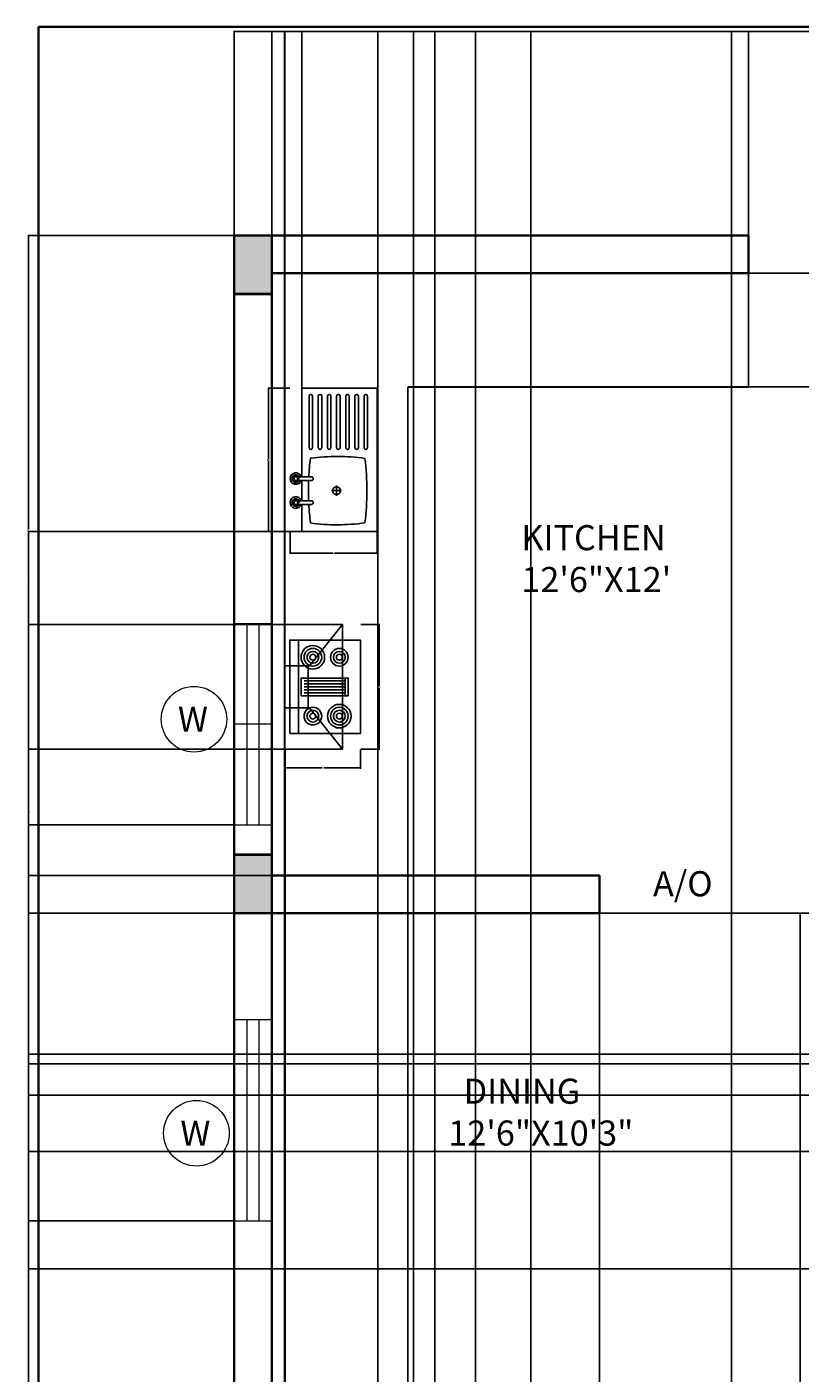
# Model space of a CAD drawing. Units: inches. Extents: x 2243 to 2668, y 14541 to 15226.
# Tile 3 of 5: x 2243 to 2428, y 14904 to 15226. Entities that reach past the tile are written whole.
import ezdxf

# ---------------------------------------------------------------- set-up
doc = ezdxf.new("R2010")
doc.units = ezdxf.units.IN
doc.header["$MEASUREMENT"] = 0
for name, color, linetype, lineweight in [('A-ANNO-DIMS', 2, 'Continuous', 18), ('A-ANNO-SYMB', 3, 'Continuous', 18), ('A-ANNO-TTLB', 7, 'Continuous', 35), ('A-AREA-IDEN', 7, 'Continuous', 18), ('A-COLS', 7, 'Continuous', 40), ('A-COLS-PATT', 7, 'Continuous', 13), ('A-EQPM', 8, 'Continuous', 25), ('A-FLOR-CASE', 9, 'Continuous', 25), ('A-FLOR-FIXT', 8, 'Continuous', 25), ('A-GLAZ', 4, 'Continuous', 18), ('A-WALL', 7, 'Continuous', 35)]:
    doc.layers.add(name, color=color, linetype=linetype, lineweight=lineweight)
doc.styles.get("Standard").update_dxf_attribs({"font": 'arial.ttf'})
doc.dimstyles.get("Standard").update_dxf_attribs({"dimtxt": 0.18, "dimasz": 0.18, "dimexe": 0.18, "dimexo": 0.0625, "dimgap": 0.09, "dimtad": 0, "dimtih": 1, "dimtoh": 1, "dimdec": 4, "dimzin": 0, "dimdsep": 46, "dimtxsty": 'Standard', "dimcen": 0.09, "dimadec": 0, "dimazin": 0, "dimtfac": 1, "dimtdec": 4, "dimtofl": 0, "dimtmove": 0, "dimatfit": 3, "dimfxl": 1, "dimtolj": 1, "dimtzin": 0, "dimarcsym": 0})

# ---------------------------------------------------------------- blocks, each defined once
blk = doc.blocks.new('chimmne')
for p, q in [((17.89, 6.07), (-18.11, 6.07)), ((-18.11, 6.07), (-18.11, -10.43)), ((-6.16, -3.43), (-18.11, 6.07)), ((5.94, -3.43), (17.89, 6.07)), ((17.89, 6.07), (17.89, -10.43)), ((-6.16, -3.43), (-6.16, -10.43)), ((5.94, -3.82), (-6.16, -3.82)), ((5.94, -3.43), (5.94, -10.43))]:
    blk.add_line(p, q)
for points in [[(-13.61, -9.12), (-13.61, 11.28), (13.39, 11.28), (13.39, -9.12)], [(-2.66, -5.87), (-2.66, 7.73), (2.44, 7.73), (2.44, -5.87)]]:
    blk.add_lwpolyline(points, close=True)
for points in [[(-2.66, 6.88), (2.44, 6.88)], [(-1.81, 6.88), (-1.81, -5.02)], [(-0.96, -5.02), (-0.96, 6.88)], [(-0.11, 6.88), (-0.11, -5.02)], [(0.74, -5.02), (0.74, 6.88)], [(1.59, 6.88), (1.59, -5.02)], [(13.39, -6.57), (-13.61, -6.57)]]:
    blk.add_lwpolyline(points)
for centre, radius in [((-8.55, 5.18), 3.4), ((-8.55, 5.18), 2.55), ((-8.55, 5.18), 1.7), ((-8.55, 5.18), 0.85), ((8.44, 5.18), 2.55), ((8.44, 5.18), 1.7), ((8.44, 5.18), 0.85), ((-8.55, -2.47), 2.55), ((8.44, -2.47), 3.4), ((8.44, -2.47), 2.55), ((-8.55, -2.47), 1.7), ((-8.55, -2.47), 0.85), ((8.44, -2.47), 1.7), ((8.44, -2.47), 0.85)]:
    blk.add_circle(centre, radius)
blk = doc.blocks.new('A$C799204C7')
for p, q in [((0, 34.2), (17.99, 34.2)), ((0, 0), (0, 34.2)), ((2.32, 20.01), (2.32, 32.27)), ((3.13, 20.01), (3.13, 32.27)), ((4.48, 20.01), (4.48, 32.27)), ((5.29, 20.01), (5.29, 32.27)), ((6.64, 20.01), (6.64, 32.27)), ((7.45, 20.01), (7.45, 32.27)), ((8.85, 20.01), (8.85, 32.27)), ((9.66, 20.01), (9.66, 32.27)), ((11.01, 20.01), (11.01, 32.27)), ((11.82, 20.01), (11.82, 32.27)), ((13.22, 20.01), (13.22, 32.27)), ((14.03, 20.01), (14.03, 32.27)), ((15.42, 20.01), (15.42, 32.27)), ((16.24, 20.01), (16.24, 32.27)), ((17.99, 13.08), (17.99, 34.2)), ((18.59, 13.08), (15.71, 13.08)), ((8.52, 9.77), (10.9, 9.77)), ((9.73, 11), (9.73, 8.54)), ((15.71, 12.17), (18.59, 12.17)), ((17.99, 7.36), (17.99, 12.17)), ((18.59, 7.36), (15.71, 7.36)), ((15.71, 6.45), (18.59, 6.45)), ((17.99, 0), (17.99, 6.45)), ((0, 0), (17.99, 0))]:
    blk.add_line(p, q)
for centre, radius in [((19.38, 12.62), 0.684), ((19.38, 12.62), 0.456), ((9.7, 9.77), 0.916), ((19.38, 6.91), 0.684), ((19.38, 6.91), 0.456)]:
    blk.add_circle(centre, radius)
for centre, radius, start, end in [((2.72, 32.27), 0.407, 0, 180), ((4.88, 32.27), 0.407, 0, 180), ((7.05, 32.27), 0.407, 0, 180), ((9.25, 32.27), 0.407, 0, 180), ((11.42, 32.27), 0.407, 0, 180), ((13.62, 32.27), 0.407, 0, 180), ((15.83, 32.27), 0.407, 0, 180), ((2.72, 20.01), 0.407, 180, 0), ((4.88, 20.01), 0.407, 180, 0), ((7.05, 20.01), 0.407, 180, 0), ((9.25, 20.01), 0.407, 180, 0), ((11.42, 20.01), 0.407, 180, 0), ((13.62, 20.01), 0.407, 180, 0), ((15.83, 20.01), 0.407, 180, 0), ((67.33, 9.77), 64.88, 173.1952, 186.8048), ((9.53, -30.19), 48.1, 82.3437, 97.8966), ((-48.51, 9.77), 64.88, 2.9208, 6.8048), ((15.71, 12.62), 0.456, 90, 270), ((19.38, 12.62), 1.37, 199.6514, 160.3603), ((19.38, 12.62), 0.911, 210.3431, 149.7554), ((-48.51, 9.77), 64.88, 357.8723, 2.115), ((15.71, 6.91), 0.456, 90, 270), ((-48.51, 9.77), 64.88, 353.1952, 357.0665), ((19.38, 6.91), 1.37, 199.6514, 160.3603), ((19.38, 6.91), 0.911, 210.3431, 149.7554), ((9.53, 49.73), 48.1, 262.1034, 277.6563)]:
    blk.add_arc(centre, radius, start, end)
blk = doc.blocks.new('WIN-48IN')
for p, q in [((0, 9), (0, 0)), ((48, 9), (0, 9)), ((48, 0), (48, 9)), ((48, 6), (0, 6)), ((0, 3), (48, 3)), ((0, 0), (48, 0))]:
    blk.add_line(p, q)
blk = doc.blocks.new('TAG-WINDOW-W')
blk.add_circle((7.84, 7.84), 7.84)
at = {"insert": (3.99, 10.84), "char_height": 6, "attachment_point": 1}
blk.add_mtext_dynamic_manual_height_columns('W', width=14.3449, gutter_width=30, heights=[0], dxfattribs=at)
blk = doc.blocks.new('*D13')
at = {"layer": 'A-ANNO-DIMS', "color": 0, "lineweight": -2, "transparency": 16777216}
for p, q in [((2323.21, 15083.13), (2327.79, 15083.13)), ((2327.61, 15082.95), (2327.61, 15068.41)), ((2327.61, 15053.5), (2327.61, 15068.04)), ((2323.21, 15053.32), (2327.79, 15053.32))]:
    blk.add_line(p, q, dxfattribs=at)
at = {"layer": 'A-ANNO-DIMS', "color": 0, "transparency": 16777216}
for points in [[(2327.58, 15082.95), (2327.64, 15082.95), (2327.61, 15083.13)], [(2327.58, 15053.5), (2327.64, 15053.5), (2327.61, 15053.32)]]:
    blk.add_solid(points, dxfattribs=at)
at = {"layer": 'Defpoints', "color": 0, "transparency": 16777216}
for p in [(2323.14, 15083.13), (2327.61, 15083.13), (2323.14, 15053.32)]:
    blk.add_point(p, dxfattribs=at)
at = {"layer": 'A-ANNO-DIMS', "color": 0, "transparency": 16777216, "insert": (2327.61, 15068.23), "char_height": 0.18, "attachment_point": 5}
blk.add_mtext('\\A1;HOB 30', dxfattribs=at)
blk = doc.blocks.new('*D14')
at = {"layer": 'A-ANNO-DIMS', "color": 0, "lineweight": -2, "transparency": 16777216}
for p, q in [((2305.17, 15053.26), (2305.17, 15048.67)), ((2323.14, 15053.26), (2323.14, 15048.67)), ((2305.35, 15048.85), (2313.95, 15048.85)), ((2322.96, 15048.85), (2314.37, 15048.85))]:
    blk.add_line(p, q, dxfattribs=at)
at = {"layer": 'A-ANNO-DIMS', "color": 0, "transparency": 16777216}
for points in [[(2305.35, 15048.88), (2305.35, 15048.82), (2305.17, 15048.85)], [(2322.96, 15048.88), (2322.96, 15048.82), (2323.14, 15048.85)]]:
    blk.add_solid(points, dxfattribs=at)
at = {"layer": 'Defpoints', "color": 0, "transparency": 16777216}
for p in [(2305.17, 15053.32), (2323.14, 15053.32), (2323.14, 15048.85)]:
    blk.add_point(p, dxfattribs=at)
at = {"layer": 'A-ANNO-DIMS', "color": 0, "transparency": 16777216, "insert": (2314.16, 15048.85), "char_height": 0.18, "attachment_point": 5}
blk.add_mtext('\\A1;18', dxfattribs=at)
blk = doc.blocks.new('*D15')
at = {"layer": 'A-ANNO-DIMS', "color": 0, "lineweight": -2, "transparency": 16777216}
for p, q in [((2306.26, 15139.64), (2301, 15139.64)), ((2301.18, 15139.46), (2301.18, 15122.67)), ((2301.18, 15105.51), (2301.18, 15122.3)), ((2306.26, 15105.33), (2301, 15105.33))]:
    blk.add_line(p, q, dxfattribs=at)
at = {"layer": 'A-ANNO-DIMS', "color": 0, "transparency": 16777216}
for points in [[(2301.15, 15139.46), (2301.21, 15139.46), (2301.18, 15139.64)], [(2301.15, 15105.51), (2301.21, 15105.51), (2301.18, 15105.33)]]:
    blk.add_solid(points, dxfattribs=at)
at = {"layer": 'Defpoints', "color": 0, "transparency": 16777216}
for p in [(2301.18, 15139.64), (2306.32, 15139.64), (2306.32, 15105.33)]:
    blk.add_point(p, dxfattribs=at)
at = {"layer": 'A-ANNO-DIMS', "color": 0, "transparency": 16777216, "insert": (2301.18, 15122.49), "char_height": 0.18, "attachment_point": 5}
blk.add_mtext('\\A1;SINK 34', dxfattribs=at)
blk = doc.blocks.new('*D16')
at = {"layer": 'A-ANNO-DIMS', "color": 0, "lineweight": -2, "transparency": 16777216}
for p, q in [((2306.32, 15105.27), (2306.32, 15100.01)), ((2327.14, 15105.27), (2327.14, 15100.01)), ((2306.5, 15100.19), (2316.53, 15100.19)), ((2326.96, 15100.19), (2316.93, 15100.19))]:
    blk.add_line(p, q, dxfattribs=at)
at = {"layer": 'A-ANNO-DIMS', "color": 0, "transparency": 16777216}
for points in [[(2306.5, 15100.22), (2306.5, 15100.16), (2306.32, 15100.19)], [(2326.96, 15100.22), (2326.96, 15100.16), (2327.14, 15100.19)]]:
    blk.add_solid(points, dxfattribs=at)
at = {"layer": 'Defpoints', "color": 0, "transparency": 16777216}
for p in [(2306.32, 15105.33), (2327.14, 15105.33), (2306.32, 15100.19)]:
    blk.add_point(p, dxfattribs=at)
at = {"layer": 'A-ANNO-DIMS', "color": 0, "transparency": 16777216, "insert": (2316.73, 15100.19), "char_height": 0.18, "attachment_point": 5}
blk.add_mtext('\\A1;21', dxfattribs=at)
blk = doc.blocks.new('*D17')
at = {"layer": 'A-ANNO-DIMS', "color": 0, "lineweight": -2, "transparency": 16777216}
for p, q in [((2292.96, 15176.2), (2292.96, 15225.04)), ((2293.14, 15224.86), (2448.67, 15224.86)), ((2604.78, 15224.86), (2449.25, 15224.86)), ((2604.96, 15176.2), (2604.96, 15225.04))]:
    blk.add_line(p, q, dxfattribs=at)
at = {"layer": 'A-ANNO-DIMS', "color": 0, "transparency": 16777216}
for points in [[(2293.14, 15224.89), (2293.14, 15224.83), (2292.96, 15224.86)], [(2604.78, 15224.89), (2604.78, 15224.83), (2604.96, 15224.86)]]:
    blk.add_solid(points, dxfattribs=at)
at = {"layer": 'Defpoints', "color": 0, "transparency": 16777216}
for p in [(2604.96, 15224.86), (2292.96, 15176.14), (2604.96, 15176.14)]:
    blk.add_point(p, dxfattribs=at)
at = {"layer": 'A-ANNO-DIMS', "color": 0, "transparency": 16777216, "insert": (2448.96, 15224.86), "char_height": 0.18, "attachment_point": 5}
blk.add_mtext('\\A1;312', dxfattribs=at)
blk = doc.blocks.new('*D25')
at = {"layer": 'A-ANNO-DIMS', "color": 0, "lineweight": -2, "transparency": 16777216}
for p, q in [((2292.9, 14940.64), (2243.57, 14940.64)), ((2243.75, 14940.46), (2243.75, 14909.07)), ((2243.75, 14877.32), (2243.75, 14908.71)), ((2292.9, 14877.14), (2243.57, 14877.14))]:
    blk.add_line(p, q, dxfattribs=at)
at = {"layer": 'A-ANNO-DIMS', "color": 0, "transparency": 16777216}
for points in [[(2243.72, 14940.46), (2243.78, 14940.46), (2243.75, 14940.64)], [(2243.72, 14877.32), (2243.78, 14877.32), (2243.75, 14877.14)]]:
    blk.add_solid(points, dxfattribs=at)
at = {"layer": 'Defpoints', "color": 0, "transparency": 16777216}
for p in [(2243.75, 14940.64), (2292.96, 14940.64), (2292.96, 14877.14)]:
    blk.add_point(p, dxfattribs=at)
at = {"layer": 'A-ANNO-DIMS', "color": 0, "transparency": 16777216, "insert": (2243.75, 14908.89), "char_height": 0.18, "attachment_point": 5}
blk.add_mtext('\\A1;63.5', dxfattribs=at)
blk = doc.blocks.new('*D26')
at = {"layer": 'A-ANNO-DIMS', "color": 0, "lineweight": -2, "transparency": 16777216}
for p, q in [((2292.9, 15014.14), (2243.57, 15014.14)), ((2243.75, 15013.96), (2243.75, 14977.57)), ((2243.75, 14940.82), (2243.75, 14977.21)), ((2292.9, 14940.64), (2243.57, 14940.64))]:
    blk.add_line(p, q, dxfattribs=at)
at = {"layer": 'A-ANNO-DIMS', "color": 0, "transparency": 16777216}
for points in [[(2243.72, 15013.96), (2243.78, 15013.96), (2243.75, 15014.14)], [(2243.72, 14940.82), (2243.78, 14940.82), (2243.75, 14940.64)]]:
    blk.add_solid(points, dxfattribs=at)
at = {"layer": 'Defpoints', "color": 0, "transparency": 16777216}
for p in [(2243.75, 15014.14), (2292.96, 15014.14), (2292.96, 14940.64)]:
    blk.add_point(p, dxfattribs=at)
at = {"layer": 'A-ANNO-DIMS', "color": 0, "transparency": 16777216, "insert": (2243.75, 14977.39), "char_height": 0.18, "attachment_point": 5}
blk.add_mtext('\\A1;73.5', dxfattribs=at)
blk = doc.blocks.new('*D27')
at = {"layer": 'A-ANNO-DIMS', "color": 0, "lineweight": -2, "transparency": 16777216}
for p, q in [((2292.9, 15035.28), (2243.57, 15035.28)), ((2243.75, 15035.1), (2243.75, 15024.89)), ((2243.75, 15014.32), (2243.75, 15024.53)), ((2292.9, 15014.14), (2243.57, 15014.14))]:
    blk.add_line(p, q, dxfattribs=at)
at = {"layer": 'A-ANNO-DIMS', "color": 0, "transparency": 16777216}
for points in [[(2243.72, 15035.1), (2243.78, 15035.1), (2243.75, 15035.28)], [(2243.72, 15014.32), (2243.78, 15014.32), (2243.75, 15014.14)]]:
    blk.add_solid(points, dxfattribs=at)
at = {"layer": 'Defpoints', "color": 0, "transparency": 16777216}
for p in [(2243.75, 15035.28), (2292.96, 15035.28), (2292.96, 15014.14)]:
    blk.add_point(p, dxfattribs=at)
at = {"layer": 'A-ANNO-DIMS', "color": 0, "transparency": 16777216, "insert": (2243.75, 15024.71), "char_height": 0.18, "attachment_point": 5}
blk.add_mtext('\\A1;21.145', dxfattribs=at)
blk = doc.blocks.new('*D28')
at = {"layer": 'A-ANNO-DIMS', "color": 0, "lineweight": -2, "transparency": 16777216}
for p, q in [((2292.9, 15176.14), (2243.57, 15176.14)), ((2243.75, 15175.96), (2243.75, 15105.89)), ((2243.75, 15035.46), (2243.75, 15105.53)), ((2292.9, 15035.28), (2243.57, 15035.28))]:
    blk.add_line(p, q, dxfattribs=at)
at = {"layer": 'A-ANNO-DIMS', "color": 0, "transparency": 16777216}
for points in [[(2243.72, 15175.96), (2243.78, 15175.96), (2243.75, 15176.14)], [(2243.72, 15035.46), (2243.78, 15035.46), (2243.75, 15035.28)]]:
    blk.add_solid(points, dxfattribs=at)
at = {"layer": 'Defpoints', "color": 0, "transparency": 16777216}
for p in [(2243.75, 15176.14), (2292.96, 15176.14), (2292.96, 15035.28)]:
    blk.add_point(p, dxfattribs=at)
at = {"layer": 'A-ANNO-DIMS', "color": 0, "transparency": 16777216, "insert": (2243.75, 15105.71), "char_height": 0.18, "attachment_point": 5}
blk.add_mtext('\\A1;140.85', dxfattribs=at)
blk = doc.blocks.new('*D31')
at = {"layer": 'A-ANNO-DIMS', "color": 0, "lineweight": -2, "transparency": 16777216}
for p, q in [((2595.9, 14980.42), (2243.57, 14980.42)), ((2243.75, 14980.24), (2243.75, 14975.71)), ((2243.75, 14970.82), (2243.75, 14975.34)), ((2595.9, 14970.64), (2243.57, 14970.64))]:
    blk.add_line(p, q, dxfattribs=at)
at = {"layer": 'A-ANNO-DIMS', "color": 0, "transparency": 16777216}
for points in [[(2243.72, 14980.24), (2243.78, 14980.24), (2243.75, 14980.42)], [(2243.72, 14970.82), (2243.78, 14970.82), (2243.75, 14970.64)]]:
    blk.add_solid(points, dxfattribs=at)
at = {"layer": 'Defpoints', "color": 0, "transparency": 16777216}
for p in [(2243.75, 14980.42), (2595.96, 14980.42), (2595.96, 14970.64)]:
    blk.add_point(p, dxfattribs=at)
at = {"layer": 'A-ANNO-DIMS', "color": 0, "transparency": 16777216, "insert": (2243.75, 14975.53), "char_height": 0.18, "attachment_point": 5}
blk.add_mtext('\\A1;9.78', dxfattribs=at)
blk = doc.blocks.new('*D32')
at = {"layer": 'A-ANNO-DIMS', "color": 0, "lineweight": -2, "transparency": 16777216}
for p, q in [((2301.96, 14673.7), (2301.96, 15225.04)), ((2302.14, 15224.86), (2303.31, 15224.86)), ((2304.78, 15224.86), (2303.61, 15224.86)), ((2304.96, 14673.7), (2304.96, 15225.04))]:
    blk.add_line(p, q, dxfattribs=at)
at = {"layer": 'A-ANNO-DIMS', "color": 0, "transparency": 16777216}
for points in [[(2302.14, 15224.89), (2302.14, 15224.83), (2301.96, 15224.86)], [(2304.78, 15224.89), (2304.78, 15224.83), (2304.96, 15224.86)]]:
    blk.add_solid(points, dxfattribs=at)
at = {"layer": 'Defpoints', "color": 0, "transparency": 16777216}
for p in [(2304.96, 15224.86), (2301.96, 14673.64), (2304.96, 14673.64)]:
    blk.add_point(p, dxfattribs=at)
at = {"layer": 'A-ANNO-DIMS', "color": 0, "transparency": 16777216, "insert": (2303.46, 15224.86), "char_height": 0.18, "attachment_point": 5}
blk.add_mtext('\\A1;3', dxfattribs=at)
blk = doc.blocks.new('*D33')
at = {"layer": 'A-ANNO-DIMS', "color": 0, "lineweight": -2, "transparency": 16777216}
for p, q in [((2304.96, 14673.7), (2304.96, 15225.04)), ((2305.14, 15224.86), (2322.74, 15224.86)), ((2340.78, 15224.86), (2323.18, 15224.86)), ((2340.96, 14673.7), (2340.96, 15225.04))]:
    blk.add_line(p, q, dxfattribs=at)
at = {"layer": 'A-ANNO-DIMS', "color": 0, "transparency": 16777216}
for points in [[(2305.14, 15224.89), (2305.14, 15224.83), (2304.96, 15224.86)], [(2340.78, 15224.89), (2340.78, 15224.83), (2340.96, 15224.86)]]:
    blk.add_solid(points, dxfattribs=at)
at = {"layer": 'Defpoints', "color": 0, "transparency": 16777216}
for p in [(2340.96, 15224.86), (2304.96, 14673.64), (2340.96, 14673.64)]:
    blk.add_point(p, dxfattribs=at)
at = {"layer": 'A-ANNO-DIMS', "color": 0, "transparency": 16777216, "insert": (2322.96, 15224.86), "char_height": 0.18, "attachment_point": 5}
blk.add_mtext('\\A1;36', dxfattribs=at)
blk = doc.blocks.new('*D34')
at = {"layer": 'A-ANNO-DIMS', "color": 0, "lineweight": -2, "transparency": 16777216}
for p, q in [((2340.96, 14673.7), (2340.96, 15225.04)), ((2341.14, 15224.86), (2352.03, 15224.86)), ((2363.71, 15224.86), (2352.82, 15224.86)), ((2363.89, 14673.7), (2363.89, 15225.04))]:
    blk.add_line(p, q, dxfattribs=at)
at = {"layer": 'A-ANNO-DIMS', "color": 0, "transparency": 16777216}
for points in [[(2341.14, 15224.89), (2341.14, 15224.83), (2340.96, 15224.86)], [(2363.71, 15224.89), (2363.71, 15224.83), (2363.89, 15224.86)]]:
    blk.add_solid(points, dxfattribs=at)
at = {"layer": 'Defpoints', "color": 0, "transparency": 16777216}
for p in [(2363.89, 15224.86), (2340.96, 14673.64), (2363.89, 14673.64)]:
    blk.add_point(p, dxfattribs=at)
at = {"layer": 'A-ANNO-DIMS', "color": 0, "transparency": 16777216, "insert": (2352.43, 15224.86), "char_height": 0.18, "attachment_point": 5}
blk.add_mtext('\\A1;22.93', dxfattribs=at)
blk = doc.blocks.new('*D35')
at = {"layer": 'A-ANNO-DIMS', "color": 0, "lineweight": -2, "transparency": 16777216}
for p, q in [((2411.89, 14673.7), (2411.89, 15225.04)), ((2412.07, 15224.86), (2431.53, 15224.86)), ((2451.78, 15224.86), (2432.32, 15224.86)), ((2451.96, 14673.7), (2451.96, 15225.04))]:
    blk.add_line(p, q, dxfattribs=at)
at = {"layer": 'A-ANNO-DIMS', "color": 0, "transparency": 16777216}
for points in [[(2412.07, 15224.89), (2412.07, 15224.83), (2411.89, 15224.86)], [(2451.78, 15224.89), (2451.78, 15224.83), (2451.96, 15224.86)]]:
    blk.add_solid(points, dxfattribs=at)
at = {"layer": 'Defpoints', "color": 0, "transparency": 16777216}
for p in [(2451.96, 15224.86), (2411.89, 14673.64), (2451.96, 14673.64)]:
    blk.add_point(p, dxfattribs=at)
at = {"layer": 'A-ANNO-DIMS', "color": 0, "transparency": 16777216, "insert": (2431.93, 15224.86), "char_height": 0.18, "attachment_point": 5}
blk.add_mtext('\\A1;40.07', dxfattribs=at)
blk = doc.blocks.new('*D41')
at = {"layer": 'A-ANNO-DIMS', "color": 0, "lineweight": -2, "transparency": 16777216}
for p, q in [((2415.96, 15176.2), (2415.96, 15225.04)), ((2416.14, 15224.86), (2433.74, 15224.86)), ((2451.78, 15224.86), (2434.18, 15224.86)), ((2451.96, 15176.2), (2451.96, 15225.04))]:
    blk.add_line(p, q, dxfattribs=at)
at = {"layer": 'A-ANNO-DIMS', "color": 0, "transparency": 16777216}
for points in [[(2416.14, 15224.89), (2416.14, 15224.83), (2415.96, 15224.86)], [(2451.78, 15224.89), (2451.78, 15224.83), (2451.96, 15224.86)]]:
    blk.add_solid(points, dxfattribs=at)
at = {"layer": 'Defpoints', "color": 0, "transparency": 16777216}
for p in [(2451.96, 15224.86), (2415.96, 15176.14), (2451.96, 15176.14)]:
    blk.add_point(p, dxfattribs=at)
at = {"layer": 'A-ANNO-DIMS', "color": 0, "transparency": 16777216, "insert": (2433.96, 15224.86), "char_height": 0.18, "attachment_point": 5}
blk.add_mtext('\\A1;36', dxfattribs=at)
blk = doc.blocks.new('*D42')
at = {"layer": 'A-ANNO-DIMS', "color": 0, "lineweight": -2, "transparency": 16777216}
for p, q in [((2380.28, 15014.07), (2380.28, 14545.86)), ((2428.28, 15014.07), (2428.28, 14545.86)), ((2380.46, 14546.04), (2404.06, 14546.04)), ((2428.1, 14546.04), (2404.5, 14546.04))]:
    blk.add_line(p, q, dxfattribs=at)
at = {"layer": 'A-ANNO-DIMS', "color": 0, "transparency": 16777216}
for points in [[(2380.46, 14546.07), (2380.46, 14546.01), (2380.28, 14546.04)], [(2428.1, 14546.07), (2428.1, 14546.01), (2428.28, 14546.04)]]:
    blk.add_solid(points, dxfattribs=at)
at = {"layer": 'Defpoints', "color": 0, "transparency": 16777216}
for p in [(2380.28, 15014.14), (2428.28, 15014.14), (2428.28, 14546.04)]:
    blk.add_point(p, dxfattribs=at)
at = {"layer": 'A-ANNO-DIMS', "color": 0, "transparency": 16777216, "insert": (2404.28, 14546.04), "char_height": 0.18, "attachment_point": 5}
blk.add_mtext('\\A1;48', dxfattribs=at)
blk = doc.blocks.new('*D43')
at = {"layer": 'A-ANNO-DIMS', "color": 0, "lineweight": -2, "transparency": 16777216}
for p, q in [((2301.96, 15023.07), (2301.96, 14545.86)), ((2334.46, 15023.07), (2334.46, 14545.86)), ((2302.14, 14546.04), (2317.89, 14546.04)), ((2334.28, 14546.04), (2318.54, 14546.04))]:
    blk.add_line(p, q, dxfattribs=at)
at = {"layer": 'A-ANNO-DIMS', "color": 0, "transparency": 16777216}
for points in [[(2302.14, 14546.07), (2302.14, 14546.01), (2301.96, 14546.04)], [(2334.28, 14546.07), (2334.28, 14546.01), (2334.46, 14546.04)]]:
    blk.add_solid(points, dxfattribs=at)
at = {"layer": 'Defpoints', "color": 0, "transparency": 16777216}
for p in [(2301.96, 15023.14), (2334.46, 15023.14), (2334.46, 14546.04)]:
    blk.add_point(p, dxfattribs=at)
at = {"layer": 'A-ANNO-DIMS', "color": 0, "transparency": 16777216, "insert": (2318.21, 14546.04), "char_height": 0.18, "attachment_point": 5}
blk.add_mtext('\\A1;32.5', dxfattribs=at)
blk = doc.blocks.new('*D44')
at = {"layer": 'A-ANNO-DIMS', "color": 0, "lineweight": -2, "transparency": 16777216}
for p, q in [((2302.02, 15167.14), (2653.58, 15167.14)), ((2653.4, 15166.96), (2653.4, 15153.7)), ((2653.4, 15140.08), (2653.4, 15153.34)), ((2334.52, 15139.9), (2653.58, 15139.9))]:
    blk.add_line(p, q, dxfattribs=at)
at = {"layer": 'A-ANNO-DIMS', "color": 0, "transparency": 16777216}
for points in [[(2653.37, 15166.96), (2653.43, 15166.96), (2653.4, 15167.14)], [(2653.37, 15140.08), (2653.43, 15140.08), (2653.4, 15139.9)]]:
    blk.add_solid(points, dxfattribs=at)
at = {"layer": 'Defpoints', "color": 0, "transparency": 16777216}
for p in [(2301.96, 15167.14), (2653.4, 15167.14), (2334.46, 15139.9)]:
    blk.add_point(p, dxfattribs=at)
at = {"layer": 'A-ANNO-DIMS', "color": 0, "transparency": 16777216, "insert": (2653.4, 15153.52), "char_height": 0.18, "attachment_point": 5}
blk.add_mtext('\\A1;27.24', dxfattribs=at)
blk = doc.blocks.new('*D45')
at = {"layer": 'A-ANNO-DIMS', "color": 0, "lineweight": -2, "transparency": 16777216}
for p, q in [((2305.11, 15053.32), (2243.57, 15053.32)), ((2243.75, 15053.14), (2243.75, 15038.41)), ((2243.75, 15023.32), (2243.75, 15038.05)), ((2301.9, 15023.14), (2243.57, 15023.14))]:
    blk.add_line(p, q, dxfattribs=at)
at = {"layer": 'A-ANNO-DIMS', "color": 0, "transparency": 16777216}
for points in [[(2243.72, 15053.14), (2243.78, 15053.14), (2243.75, 15053.32)], [(2243.72, 15023.32), (2243.78, 15023.32), (2243.75, 15023.14)]]:
    blk.add_solid(points, dxfattribs=at)
at = {"layer": 'Defpoints', "color": 0, "transparency": 16777216}
for p in [(2243.75, 15053.32), (2305.17, 15053.32), (2301.96, 15023.14)]:
    blk.add_point(p, dxfattribs=at)
at = {"layer": 'A-ANNO-DIMS', "color": 0, "transparency": 16777216, "insert": (2243.75, 15038.23), "char_height": 0.18, "attachment_point": 5}
blk.add_mtext('\\A1;30.184', dxfattribs=at)
blk = doc.blocks.new('*D46')
at = {"layer": 'A-ANNO-DIMS', "color": 0, "lineweight": -2, "transparency": 16777216}
for p, q in [((2309.03, 15105.33), (2243.57, 15105.33)), ((2243.75, 15105.15), (2243.75, 15094.41)), ((2243.75, 15083.31), (2243.75, 15094.05)), ((2305.11, 15083.13), (2243.57, 15083.13))]:
    blk.add_line(p, q, dxfattribs=at)
at = {"layer": 'A-ANNO-DIMS', "color": 0, "transparency": 16777216}
for points in [[(2243.72, 15105.15), (2243.78, 15105.15), (2243.75, 15105.33)], [(2243.72, 15083.31), (2243.78, 15083.31), (2243.75, 15083.13)]]:
    blk.add_solid(points, dxfattribs=at)
at = {"layer": 'Defpoints', "color": 0, "transparency": 16777216}
for p in [(2243.75, 15105.33), (2309.09, 15105.33), (2305.17, 15083.13)]:
    blk.add_point(p, dxfattribs=at)
at = {"layer": 'A-ANNO-DIMS', "color": 0, "transparency": 16777216, "insert": (2243.75, 15094.23), "char_height": 0.18, "attachment_point": 5}
blk.add_mtext('\\A1;22.203', dxfattribs=at)
blk = doc.blocks.new('*D51')
at = {"layer": 'A-ANNO-DIMS', "color": 0, "lineweight": -2, "transparency": 16777216}
for p, q in [((2531.4, 14929.14), (2243.57, 14929.14)), ((2243.75, 14928.96), (2243.75, 14913.32)), ((2243.75, 14897.32), (2243.75, 14912.95)), ((2531.4, 14897.14), (2243.57, 14897.14))]:
    blk.add_line(p, q, dxfattribs=at)
at = {"layer": 'A-ANNO-DIMS', "color": 0, "transparency": 16777216}
for points in [[(2243.72, 14928.96), (2243.78, 14928.96), (2243.75, 14929.14)], [(2243.72, 14897.32), (2243.78, 14897.32), (2243.75, 14897.14)]]:
    blk.add_solid(points, dxfattribs=at)
at = {"layer": 'Defpoints', "color": 0, "transparency": 16777216}
for p in [(2243.75, 14929.14), (2531.46, 14929.14), (2531.46, 14897.14)]:
    blk.add_point(p, dxfattribs=at)
at = {"layer": 'A-ANNO-DIMS', "color": 0, "transparency": 16777216, "insert": (2243.75, 14913.14), "char_height": 0.18, "attachment_point": 5}
blk.add_mtext('\\A1;32', dxfattribs=at)
blk = doc.blocks.new('*D53')
at = {"layer": 'A-ANNO-DIMS', "color": 0, "lineweight": -2, "transparency": 16777216}
for p, q in [((2451.9, 15014.14), (2243.57, 15014.14)), ((2243.75, 15013.96), (2243.75, 14996.32)), ((2243.75, 14978.32), (2243.75, 14995.95)), ((2451.9, 14978.14), (2243.57, 14978.14))]:
    blk.add_line(p, q, dxfattribs=at)
at = {"layer": 'A-ANNO-DIMS', "color": 0, "transparency": 16777216}
for points in [[(2243.72, 15013.96), (2243.78, 15013.96), (2243.75, 15014.14)], [(2243.72, 14978.32), (2243.78, 14978.32), (2243.75, 14978.14)]]:
    blk.add_solid(points, dxfattribs=at)
at = {"layer": 'Defpoints', "color": 0, "transparency": 16777216}
for p in [(2243.75, 15014.14), (2451.96, 15014.14), (2451.96, 14978.14)]:
    blk.add_point(p, dxfattribs=at)
at = {"layer": 'A-ANNO-DIMS', "color": 0, "transparency": 16777216, "insert": (2243.75, 14996.14), "char_height": 0.18, "attachment_point": 5}
blk.add_mtext('\\A1;36', dxfattribs=at)
blk = doc.blocks.new('*D54')
at = {"layer": 'A-ANNO-DIMS', "color": 0, "lineweight": -2, "transparency": 16777216}
for p, q in [((2451.9, 14957.21), (2243.57, 14957.21)), ((2243.75, 14957.03), (2243.75, 14927.48)), ((2243.75, 14897.56), (2243.75, 14927.11)), ((2451.9, 14897.38), (2243.57, 14897.38))]:
    blk.add_line(p, q, dxfattribs=at)
at = {"layer": 'A-ANNO-DIMS', "color": 0, "transparency": 16777216}
for points in [[(2243.72, 14957.03), (2243.78, 14957.03), (2243.75, 14957.21)], [(2243.72, 14897.56), (2243.78, 14897.56), (2243.75, 14897.38)]]:
    blk.add_solid(points, dxfattribs=at)
at = {"layer": 'Defpoints', "color": 0, "transparency": 16777216}
for p in [(2243.75, 14957.21), (2451.96, 14957.21), (2451.96, 14897.38)]:
    blk.add_point(p, dxfattribs=at)
at = {"layer": 'A-ANNO-DIMS', "color": 0, "transparency": 16777216, "insert": (2243.75, 14927.3), "char_height": 0.18, "attachment_point": 5}
blk.add_mtext('\\A1;59.83', dxfattribs=at)
blk = doc.blocks.new('*D56')
at = {"layer": 'A-ANNO-DIMS', "color": 0, "lineweight": -2, "transparency": 16777216}
for p, q in [((2305.04, 14786.87), (2305.04, 15225.04)), ((2305.22, 15224.86), (2315.76, 15224.86)), ((2327.09, 15224.86), (2316.55, 15224.86)), ((2327.27, 14788.83), (2327.27, 15225.04))]:
    blk.add_line(p, q, dxfattribs=at)
at = {"layer": 'A-ANNO-DIMS', "color": 0, "transparency": 16777216}
for points in [[(2305.22, 15224.89), (2305.22, 15224.83), (2305.04, 15224.86)], [(2327.09, 15224.89), (2327.09, 15224.83), (2327.27, 15224.86)]]:
    blk.add_solid(points, dxfattribs=at)
at = {"layer": 'Defpoints', "color": 0, "transparency": 16777216}
for p in [(2327.27, 15224.86), (2305.04, 14786.81), (2327.27, 14788.77)]:
    blk.add_point(p, dxfattribs=at)
at = {"layer": 'A-ANNO-DIMS', "color": 0, "transparency": 16777216, "insert": (2316.15, 15224.86), "char_height": 0.18, "attachment_point": 5}
blk.add_mtext('\\A1;22.23', dxfattribs=at)
blk = doc.blocks.new('*D59')
at = {"layer": 'A-ANNO-DIMS', "color": 0, "lineweight": -2, "transparency": 16777216}
for p, q in [((2335.83, 14775.7), (2335.83, 15225.04)), ((2336.01, 15224.86), (2342.78, 15224.86)), ((2350.47, 15224.86), (2343.69, 15224.86)), ((2350.65, 14775.7), (2350.65, 15225.04))]:
    blk.add_line(p, q, dxfattribs=at)
at = {"layer": 'A-ANNO-DIMS', "color": 0, "transparency": 16777216}
for points in [[(2336.01, 15224.89), (2336.01, 15224.83), (2335.83, 15224.86)], [(2350.47, 15224.89), (2350.47, 15224.83), (2350.65, 15224.86)]]:
    blk.add_solid(points, dxfattribs=at)
at = {"layer": 'Defpoints', "color": 0, "transparency": 16777216}
for p in [(2350.65, 15224.86), (2335.83, 14775.64), (2350.65, 14775.64)]:
    blk.add_point(p, dxfattribs=at)
at = {"layer": 'A-ANNO-DIMS', "color": 0, "transparency": 16777216, "insert": (2343.24, 15224.86), "char_height": 0.18, "attachment_point": 5}
blk.add_mtext('\\A1;14.818', dxfattribs=at)
blk = doc.blocks.new('*D61')
at = {"layer": 'A-ANNO-DIMS', "color": 0, "lineweight": -2, "transparency": 16777216}
for p, q in [((2301.96, 15023.07), (2301.96, 14545.86)), ((2380.28, 15014.07), (2380.28, 14545.86)), ((2302.14, 14546.04), (2340.73, 14546.04)), ((2380.1, 14546.04), (2341.51, 14546.04))]:
    blk.add_line(p, q, dxfattribs=at)
at = {"layer": 'A-ANNO-DIMS', "color": 0, "transparency": 16777216}
for points in [[(2302.14, 14546.07), (2302.14, 14546.01), (2301.96, 14546.04)], [(2380.1, 14546.07), (2380.1, 14546.01), (2380.28, 14546.04)]]:
    blk.add_solid(points, dxfattribs=at)
at = {"layer": 'Defpoints', "color": 0, "transparency": 16777216}
for p in [(2301.96, 15023.14), (2380.28, 15014.14), (2380.28, 14546.04)]:
    blk.add_point(p, dxfattribs=at)
at = {"layer": 'A-ANNO-DIMS', "color": 0, "transparency": 16777216, "insert": (2341.12, 14546.04), "char_height": 0.18, "attachment_point": 5}
blk.add_mtext('\\A1;78.32', dxfattribs=at)
blk = doc.blocks.new('*D65')
at = {"layer": 'A-ANNO-DIMS', "color": 0, "lineweight": -2, "transparency": 16777216}
for p, q in [((2305.17, 15053.26), (2305.17, 14545.86)), ((2301.96, 15035.22), (2301.96, 14545.86)), ((2302.14, 14546.04), (2303.26, 14546.04)), ((2304.99, 14546.04), (2303.87, 14546.04))]:
    blk.add_line(p, q, dxfattribs=at)
at = {"layer": 'A-ANNO-DIMS', "color": 0, "transparency": 16777216}
for points in [[(2302.14, 14546.07), (2302.14, 14546.01), (2301.96, 14546.04)], [(2304.99, 14546.07), (2304.99, 14546.01), (2305.17, 14546.04)]]:
    blk.add_solid(points, dxfattribs=at)
at = {"layer": 'Defpoints', "color": 0, "transparency": 16777216}
for p in [(2305.17, 15053.32), (2301.96, 15035.28), (2305.17, 14546.04)]:
    blk.add_point(p, dxfattribs=at)
at = {"layer": 'A-ANNO-DIMS', "color": 0, "transparency": 16777216, "insert": (2303.56, 14546.04), "char_height": 0.18, "attachment_point": 5}
blk.add_mtext('\\A1;3.21', dxfattribs=at)
blk = doc.blocks.new('*D66')
at = {"layer": 'A-ANNO-DIMS', "color": 0, "lineweight": -2, "transparency": 16777216}
for p, q in [((2301.96, 15167.2), (2301.96, 15225.04)), ((2302.14, 15224.86), (2305.13, 15224.86)), ((2308.91, 15224.86), (2305.92, 15224.86)), ((2309.09, 15139.71), (2309.09, 15225.04))]:
    blk.add_line(p, q, dxfattribs=at)
at = {"layer": 'A-ANNO-DIMS', "color": 0, "transparency": 16777216}
for points in [[(2302.14, 15224.89), (2302.14, 15224.83), (2301.96, 15224.86)], [(2308.91, 15224.89), (2308.91, 15224.83), (2309.09, 15224.86)]]:
    blk.add_solid(points, dxfattribs=at)
at = {"layer": 'Defpoints', "color": 0, "transparency": 16777216}
for p in [(2309.09, 15224.86), (2301.96, 15167.14), (2309.09, 15139.64)]:
    blk.add_point(p, dxfattribs=at)
at = {"layer": 'A-ANNO-DIMS', "color": 0, "transparency": 16777216, "insert": (2305.52, 15224.86), "char_height": 0.18, "attachment_point": 5}
blk.add_mtext('\\A1;7.128', dxfattribs=at)

msp = doc.modelspace()

# ---------------------------------------------------------------- hatches: boundary and pattern name
at = {"layer": 'A-COLS-PATT'}
h = msp.add_hatch(color=256, dxfattribs=at)
h.dxf.hatch_style = 1
h.paths.add_polyline_path([(2301.96, 15176.1368), (2292.96, 15176.1368), (2292.96, 15162.1368), (2301.96, 15162.1368)])
h.paths.add_polyline_path([(2460.96, 15176.1368), (2451.96, 15176.1368), (2451.96, 15162.1368), (2460.96, 15162.1368)])
h.paths.add_polyline_path([(2604.96, 15176.1368), (2595.96, 15176.1368), (2595.96, 15162.1368), (2604.96, 15162.1368)])
h.paths.add_polyline_path([(2301.96, 15028.1368), (2292.96, 15028.1368), (2292.96, 15014.1368), (2301.96, 15014.1368)])
h.paths.add_polyline_path([(2460.96, 15028.1368), (2451.96, 15028.1368), (2451.96, 15014.1368), (2460.96, 15014.1368)])
h.paths.add_polyline_path([(2604.96, 15027.8868), (2595.96, 15027.8868), (2595.96, 15013.8868), (2604.96, 15013.8868)])
h.paths.add_polyline_path([(2301.96, 14891.1368), (2292.96, 14891.1368), (2292.96, 14877.1368), (2301.96, 14877.1368)])
h.paths.add_polyline_path([(2460.96, 14891.1368), (2451.96, 14891.1368), (2451.96, 14877.1368), (2460.96, 14877.1368)])
h.paths.add_polyline_path([(2604.96, 14891.1368), (2595.96, 14891.1368), (2595.96, 14877.1368), (2604.96, 14877.1368)])
h.paths.add_polyline_path([(2301.96, 14678.6368), (2292.96, 14678.6368), (2292.96, 14664.6368), (2301.96, 14664.6368)])
h.paths.add_polyline_path([(2460.96, 14678.6368), (2451.96, 14678.6368), (2451.96, 14664.6368), (2460.96, 14664.6368)])
h.paths.add_polyline_path([(2604.96, 14678.6368), (2595.96, 14678.6368), (2595.96, 14664.6368), (2604.96, 14664.6368)])
h.paths.add_polyline_path([(2604.96, 14591.6368), (2595.96, 14591.6368), (2595.96, 14577.6368), (2604.96, 14577.6368)])
h.paths.add_polyline_path([(2460.96, 14591.6368), (2451.96, 14591.6368), (2451.96, 14577.6368), (2460.96, 14577.6368)])
h.paths.add_polyline_path([(2306.96, 14586.6368), (2292.96, 14586.6368), (2292.96, 14577.6368), (2306.96, 14577.6368)])

# ---------------------------------------------------------------- linework, layer by layer
at = {"layer": 'A-ANNO-TTLB'}
msp.add_lwpolyline([(2246.1122, 15225.9536), (2667.5226, 15225.9536), (2667.5226, 14540.814), (2246.1122, 14540.814)], close=True, dxfattribs=at)
at = {"layer": 'A-COLS'}
for p, q in [((2292.96, 15162.1368), (2301.96, 15162.1368)), ((2292.96, 15028.1368), (2301.96, 15028.1368))]:
    msp.add_line(p, q, dxfattribs=at)
at = {"layer": 'A-FLOR-CASE'}
for p, q in [((2415.96, 15167.1368), (2415.96, 15139.8973)), ((2415.96, 15139.8973), (2334.4616, 15139.8973)), ((2334.4616, 15139.8973), (2334.4616, 15023.1368))]:
    msp.add_line(p, q, dxfattribs=at)
at = {"layer": 'A-GLAZ'}
msp.add_line((2301.96, 15059.282), (2292.96, 15059.282), dxfattribs=at)
at = {"layer": 'A-WALL'}
for p, q in [((2292.96, 15176.1368), (2415.96, 15176.1368)), ((2292.96, 15176.1368), (2292.96, 14577.6368)), ((2301.96, 15176.1368), (2301.96, 14586.6368)), ((2415.96, 15176.1368), (2415.96, 15167.1368)), ((2301.96, 15167.1368), (2415.96, 15167.1368)), ((2301.96, 15023.1368), (2380.2818, 15023.1368)), ((2380.2818, 15014.1368), (2380.2818, 15023.1368)), ((2292.96, 15014.1368), (2380.2818, 15014.1368))]:
    msp.add_line(p, q, dxfattribs=at)

# ---------------------------------------------------------------- block references
at = {"layer": 'A-ANNO-SYMB'}
for p in [(2275.4959, 15052.6647), (2276.0738, 14953.7063)]:
    msp.add_blockref('TAG-WINDOW-W', p, dxfattribs=at)
at = {"layer": 'A-EQPM', "xscale": -0.8280321260258986, "yscale": 0.8280321260258986, "zscale": 0.8280321260258986, "rotation": 270}
msp.add_blockref('chimmne', (2313.8058, 15068.3184), dxfattribs=at)
at = {"layer": 'A-FLOR-FIXT', "xscale": -1.0032, "yscale": 1.0032, "zscale": 1.0032}
msp.add_blockref('A$C799204C7', (2327.1374, 15105.3331), dxfattribs=at)
at = {"layer": 'A-GLAZ'}
for p, rotation in [((2292.9602, 15083.2821), 269.9999999999984), ((2301.9598, 14940.6414), 89.999999999996)]:
    msp.add_blockref('WIN-48IN', p, dxfattribs=dict(at, rotation=rotation))

# ---------------------------------------------------------------- texts
at = {"layer": 'A-ANNO-SYMB', "insert": (2393.1088, 15024.1854), "char_height": 6, "attachment_point": 1}
msp.add_mtext_dynamic_manual_height_columns('A/O', width=16.844499, gutter_width=30, heights=[0], dxfattribs=at)
at = {"layer": 'A-AREA-IDEN', "char_height": 6, "attachment_point": 1}
for s, width, insert in [('KITCHEN\\P12\'6"X12\'', 67.914475, (2361.6271, 15106.8919)), ('  DINING\\P12\'6"X10\'3"', 62.699556, (2344.1594, 14974.5964))]:
    msp.add_mtext_dynamic_manual_height_columns(s, width=width, gutter_width=30, heights=[0], dxfattribs=dict(at, insert=insert))

# ---------------------------------------------------------------- dimensions: what is measured, and where the dimension line sits
at = {"layer": 'A-ANNO-DIMS'}
for base, p1, p2, override, picture, middle in [((2604.96, 15224.8619), (2292.96, 15176.1368), (2604.96, 15176.1368), {"dimdec": 0, "dimlfac": 1, "dimrnd": 0, "dimzin": 0, "dimdsep": 46, "dimlunit": 2}, '*D17', (2448.96, 15224.8619)), ((2304.96, 15224.8619), (2301.96, 14673.6368), (2304.96, 14673.6368), {"dimdec": 0, "dimlfac": 1, "dimrnd": 0, "dimzin": 0, "dimdsep": 46, "dimlunit": 2}, '*D32', (2303.46, 15224.8619)), ((2309.0878, 15224.8619), (2301.96, 15167.1368), (2309.0878, 15139.6426), {"dimdec": 3, "dimlfac": 1, "dimrnd": 0, "dimzin": 0, "dimdsep": 46, "dimlunit": 2}, '*D66', (2305.5239, 15224.8619)), ((2340.96, 15224.8619), (2304.96, 14673.6368), (2340.96, 14673.6368), {"dimdec": 0, "dimlfac": 1, "dimrnd": 0, "dimzin": 0, "dimdsep": 46, "dimlunit": 2}, '*D33', (2322.96, 15224.8619)), ((2327.2661, 15224.8619), (2305.0371, 14786.8054), (2327.2661, 14788.7668), {"dimdec": 2, "dimlfac": 1, "dimrnd": 0, "dimzin": 0, "dimdsep": 46, "dimlunit": 2}, '*D56', (2316.1516, 15224.8619)), ((2350.6465, 15224.8619), (2335.8284, 14775.637), (2350.6465, 14775.637), {"dimdec": 3, "dimlfac": 1, "dimrnd": 0, "dimzin": 0, "dimdsep": 46, "dimlunit": 2}, '*D59', (2343.2375, 15224.8619)), ((2363.8914, 15224.8619), (2340.96, 14673.6368), (2363.8914, 14673.6368), {"dimdec": 2, "dimlfac": 1, "dimrnd": 0, "dimzin": 0, "dimdsep": 46, "dimlunit": 2}, '*D34', (2352.4257, 15224.8619)), ((2451.96, 15224.8619), (2411.8914, 14673.6368), (2451.96, 14673.6368), {"dimdec": 2, "dimlfac": 1, "dimrnd": 0, "dimzin": 0, "dimdsep": 46, "dimlunit": 2}, '*D35', (2431.9257, 15224.8619)), ((2451.96, 15224.8619), (2415.96, 15176.1368), (2451.96, 15176.1368), {"dimdec": 0, "dimlfac": 1, "dimrnd": 0, "dimzin": 0, "dimdsep": 46, "dimlunit": 2}, '*D41', (2433.96, 15224.8619)), ((2305.1696, 14546.0368), (2301.96, 15035.282), (2305.1696, 15053.321), {"dimdec": 2, "dimlfac": 1, "dimrnd": 0, "dimzin": 0, "dimdsep": 46, "dimlunit": 2}, '*D65', (2303.5648, 14546.0368)), ((2323.1431, 15048.8496), (2305.1696, 15053.321), (2323.1431, 15053.321), {"dimdec": 0, "dimlfac": 1, "dimrnd": 0, "dimzin": 0, "dimdsep": 46, "dimlunit": 2}, '*D14', (2314.1564, 15048.8496)), ((2334.4616, 14546.0368), (2301.96, 15023.1368), (2334.4616, 15023.1368), {"dimdec": 1, "dimlfac": 1, "dimrnd": 0, "dimzin": 0, "dimdsep": 46, "dimlunit": 2}, '*D43', (2318.2108, 14546.0368)), ((2380.2818, 14546.0368), (2301.96, 15023.1368), (2380.2818, 15014.1368), {"dimdec": 2, "dimlfac": 1, "dimrnd": 0, "dimzin": 0, "dimdsep": 46, "dimlunit": 2}, '*D61', (2341.1209, 14546.0368)), ((2428.2818, 14546.0368), (2380.2818, 15014.1368), (2428.2818, 15014.1368), {"dimdec": 0, "dimlfac": 1, "dimrnd": 0, "dimzin": 0, "dimdsep": 46, "dimlunit": 2}, '*D42', (2404.2818, 14546.0368))]:
    dim = msp.add_linear_dim(base=base, p1=p1, p2=p2, dimstyle='Standard', override=override, dxfattribs=at)
    dim.commit()
    dim.dimension.update_dxf_attribs({"geometry": picture, "text_midpoint": middle})
for base, p1, p2, angle, override, picture, middle in [((2243.7531, 15176.1368), (2292.96, 15035.282), (2292.96, 15176.1368), 90, {"dimdec": 2, "dimlfac": 1, "dimrnd": 0, "dimzin": 0, "dimdsep": 46, "dimlunit": 2}, '*D28', (2243.7531, 15105.7094)), ((2653.4036, 15167.1368), (2334.4616, 15139.8973), (2301.96, 15167.1368), 90, {"dimdec": 2, "dimlfac": 1, "dimrnd": 0, "dimzin": 0, "dimdsep": 46, "dimlunit": 2}, '*D44', (2653.4036, 15153.5171)), ((2243.7531, 15105.3331), (2305.1696, 15083.1302), (2309.0878, 15105.3331), 90, {"dimdec": 3, "dimlfac": 1, "dimrnd": 0, "dimzin": 0, "dimdsep": 46, "dimlunit": 2}, '*D46', (2243.7531, 15094.2317)), ((2306.3233, 15100.1867), (2327.1374, 15105.3331), (2306.3233, 15105.3331), 180, {"dimdec": 0, "dimlfac": 1, "dimrnd": 0, "dimzin": 0, "dimdsep": 46, "dimlunit": 2}, '*D16', (2316.7303, 15100.1867)), ((2243.7531, 15053.321), (2301.96, 15023.1368), (2305.1696, 15053.321), 90, {"dimdec": 3, "dimlfac": 1, "dimrnd": 0, "dimzin": 0, "dimdsep": 46, "dimlunit": 2}, '*D45', (2243.7531, 15038.2289)), ((2243.7531, 15035.282), (2292.96, 15014.1368), (2292.96, 15035.282), 90, {"dimdec": 3, "dimlfac": 1, "dimrnd": 0, "dimzin": 0, "dimdsep": 46, "dimlunit": 2}, '*D27', (2243.7531, 15024.7094)), ((2243.7531, 15014.1368), (2292.96, 14940.6414), (2292.96, 15014.1368), 90, {"dimdec": 1, "dimlfac": 1, "dimrnd": 0, "dimzin": 0, "dimdsep": 46, "dimlunit": 2}, '*D26', (2243.7531, 14977.3891)), ((2243.7531, 15014.1368), (2451.96, 14978.1368), (2451.96, 15014.1368), 90, {"dimdec": 0, "dimlfac": 1, "dimrnd": 0, "dimzin": 0, "dimdsep": 46, "dimlunit": 2}, '*D53', (2243.7531, 14996.1368)), ((2243.7531, 14980.4164), (2595.96, 14970.6368), (2595.96, 14980.4164), 90, {"dimdec": 2, "dimlfac": 1, "dimrnd": 0, "dimzin": 0, "dimdsep": 46, "dimlunit": 2}, '*D31', (2243.7531, 14975.5266)), ((2243.7531, 14957.2115), (2451.96, 14897.3823), (2451.96, 14957.2115), 90, {"dimdec": 2, "dimlfac": 1, "dimrnd": 0, "dimzin": 0, "dimdsep": 46, "dimlunit": 2}, '*D54', (2243.7531, 14927.2969)), ((2243.7531, 14940.6414), (2292.96, 14877.1368), (2292.96, 14940.6414), 90, {"dimdec": 1, "dimlfac": 1, "dimrnd": 0, "dimzin": 0, "dimdsep": 46, "dimlunit": 2}, '*D25', (2243.7531, 14908.8891)), ((2243.7531, 14929.1368), (2531.46, 14897.1368), (2531.46, 14929.1368), 90, {"dimdec": 0, "dimlfac": 1, "dimrnd": 0, "dimzin": 0, "dimdsep": 46, "dimlunit": 2}, '*D51', (2243.7531, 14913.1368))]:
    dim = msp.add_linear_dim(base=base, p1=p1, p2=p2, angle=angle, dimstyle='Standard', override=override, dxfattribs=at)
    dim.commit()
    dim.dimension.update_dxf_attribs({"geometry": picture, "text_midpoint": middle})
for base, p1, p2, text, picture, middle in [((2301.1769, 15139.6426), (2306.3233, 15105.3331), (2306.3233, 15139.6426), 'SINK <>', '*D15', (2301.1769, 15122.4879)), ((2327.6145, 15083.1302), (2323.1431, 15053.321), (2323.1431, 15083.1302), 'HOB <>', '*D13', (2327.6145, 15068.2256))]:
    dim = msp.add_linear_dim(base=base, p1=p1, p2=p2, angle=90, text=text, dimstyle='Standard', override={"dimdec": 0, "dimlfac": 1, "dimrnd": 0, "dimzin": 0, "dimdsep": 46, "dimlunit": 2}, dxfattribs=at)
    dim.commit()
    dim.dimension.update_dxf_attribs({"geometry": picture, "text_midpoint": middle})

doc.saveas('drawing.dxf')
